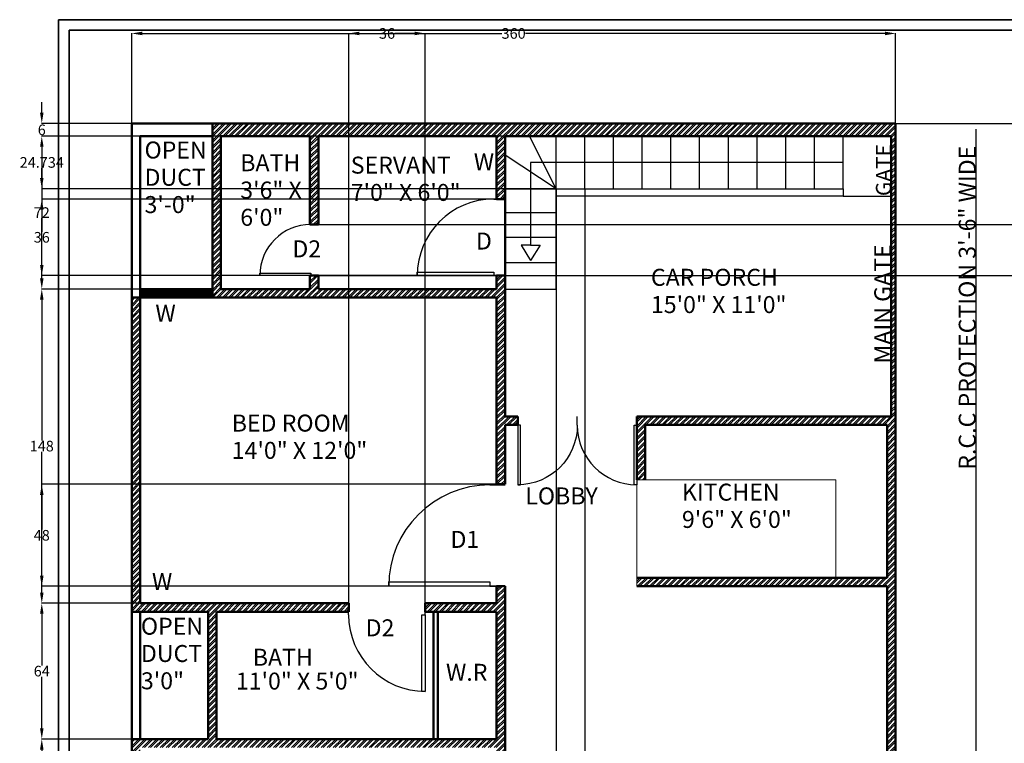
# Model space of a CAD drawing. Units: inches. Extents: x -35 to 905, y -602 to 298.
# Tile 2 of 4: x -35 to 429, y -43 to 298. Entities that reach past the tile are written whole.
import ezdxf

# ---------------------------------------------------------------- set-up
doc = ezdxf.new("R2010")
doc.units = ezdxf.units.IN
doc.header["$MEASUREMENT"] = 0
for name, color, linetype, lineweight in [('A-ANNO-DIMS', 2, 'Continuous', 18), ('A-ANNO-TEXT', 3, 'Continuous', 18), ('A-ANNO-TTLB', 7, 'Continuous', 35), ('A-AREA-IDEN', 7, 'Continuous', 18), ('A-DOOR', 4, 'Continuous', 25), ('A-FLOR-FIXT', 8, 'Continuous', 18), ('A-FLOR-STRS', 3, 'Continuous', 25), ('A-WALL', 7, 'Continuous', 50), ('A-WALL-PATT', 8, 'Continuous', 13), ('C-PROP', 1, 'Continuous', 25)]:
    doc.layers.add(name, color=color, linetype=linetype, lineweight=lineweight)
doc.styles.get("Standard").update_dxf_attribs({"font": 'arial.ttf'})
doc.dimstyles.get("Standard").update_dxf_attribs({"dimtxt": 5, "dimasz": 5, "dimexe": 0.18, "dimexo": 0.0625, "dimgap": 0.09, "dimtad": 0, "dimtih": 1, "dimtoh": 1, "dimdec": 1, "dimzin": 0, "dimdsep": 46, "dimlunit": 4, "dimtxsty": 'Standard', "dimcen": 0.09, "dimadec": 0, "dimazin": 0, "dimtfac": 1, "dimtdec": 1, "dimtofl": 0, "dimtmove": 0, "dimatfit": 3, "dimfxl": 1, "dimtolj": 1, "dimtzin": 0, "dimarcsym": 0})

# ---------------------------------------------------------------- blocks, each defined once
blk = doc.blocks.new('*U2')
for p, q in [((0, 0), (0, -6)), ((40, 0), (40, -6))]:
    blk.add_line(p, q)
blk.add_lwpolyline([(0, 0), (0, 40), (1.75, 40), (1.75, 0)], close=True)
blk.add_arc((0, 0), 40, 0, 90)
blk = doc.blocks.new('*D3')
at = {"layer": 'A-ANNO-DIMS', "color": 0, "lineweight": -2, "ltscale": 0.3, "transparency": 16777216}
for p, q in [((17.78, 249.41), (17.78, 291.93)), ((22.78, 291.75), (192.18, 291.75)), ((372.78, 291.75), (203.39, 291.75)), ((377.78, 249.41), (377.78, 291.93))]:
    blk.add_line(p, q, dxfattribs=at)
at = {"layer": 'A-ANNO-DIMS', "color": 0, "ltscale": 0.3, "transparency": 16777216}
for points in [[(22.78, 292.58), (22.78, 290.91), (17.78, 291.75)], [(372.78, 292.58), (372.78, 290.91), (377.78, 291.75)]]:
    blk.add_solid(points, dxfattribs=at)
at = {"layer": 'Defpoints', "color": 0, "ltscale": 0.3, "transparency": 16777216}
for p in [(377.78, 291.75), (17.78, 249.35), (377.78, 249.35)]:
    blk.add_point(p, dxfattribs=at)
at = {"layer": 'A-ANNO-DIMS', "color": 0, "ltscale": 0.3, "transparency": 16777216, "insert": (197.78, 291.75), "char_height": 5, "attachment_point": 5}
blk.add_mtext('\\A1;360', dxfattribs=at)
blk = doc.blocks.new('*D4')
at = {"layer": 'A-ANNO-DIMS', "color": 0, "lineweight": -2, "ltscale": 0.3, "transparency": 16777216}
for p, q in [((-24.62, 254.35), (-24.62, 259.35)), ((17.72, 249.35), (-24.8, 249.35)), ((21.72, 243.35), (-24.8, 243.35)), ((-24.62, 238.35), (-24.62, 233.35))]:
    blk.add_line(p, q, dxfattribs=at)
at = {"layer": 'A-ANNO-DIMS', "color": 0, "ltscale": 0.3, "transparency": 16777216}
for points in [[(-25.45, 254.35), (-23.78, 254.35), (-24.62, 249.35)], [(-25.45, 238.35), (-23.78, 238.35), (-24.62, 243.35)]]:
    blk.add_solid(points, dxfattribs=at)
at = {"layer": 'Defpoints', "color": 0, "ltscale": 0.3, "transparency": 16777216}
for p in [(17.78, 249.35), (-24.62, 243.35), (21.78, 243.35)]:
    blk.add_point(p, dxfattribs=at)
at = {"layer": 'A-ANNO-DIMS', "color": 0, "ltscale": 0.3, "transparency": 16777216, "insert": (-24.62, 246.35), "char_height": 5, "attachment_point": 5}
blk.add_mtext('\\A1;6', dxfattribs=at)
blk = doc.blocks.new('*D5')
at = {"layer": 'A-ANNO-DIMS', "color": 0, "lineweight": -2, "ltscale": 0.3, "transparency": 16777216}
for p, q in [((21.72, 243.35), (-24.8, 243.35)), ((-24.62, 238.35), (-24.62, 209.95)), ((-24.62, 176.35), (-24.62, 204.75)), ((21.72, 171.35), (-24.8, 171.35))]:
    blk.add_line(p, q, dxfattribs=at)
at = {"layer": 'A-ANNO-DIMS', "color": 0, "ltscale": 0.3, "transparency": 16777216}
for points in [[(-25.45, 238.35), (-23.78, 238.35), (-24.62, 243.35)], [(-25.45, 176.35), (-23.78, 176.35), (-24.62, 171.35)]]:
    blk.add_solid(points, dxfattribs=at)
at = {"layer": 'Defpoints', "color": 0, "ltscale": 0.3, "transparency": 16777216}
for p in [(21.78, 243.35), (-24.62, 171.35), (21.78, 171.35)]:
    blk.add_point(p, dxfattribs=at)
at = {"layer": 'A-ANNO-DIMS', "color": 0, "ltscale": 0.3, "transparency": 16777216, "insert": (-24.62, 207.35), "char_height": 5, "attachment_point": 5}
blk.add_mtext('\\A1;72', dxfattribs=at)
blk = doc.blocks.new('*D6')
at = {"layer": 'A-ANNO-DIMS', "color": 0, "lineweight": -2, "ltscale": 0.3, "transparency": 16777216}
for p, q in [((21.72, 171.35), (-24.8, 171.35)), ((-24.62, 166.35), (-24.62, 99.99)), ((-24.62, 28.35), (-24.62, 94.7)), ((21.72, 23.35), (-24.8, 23.35))]:
    blk.add_line(p, q, dxfattribs=at)
at = {"layer": 'A-ANNO-DIMS', "color": 0, "ltscale": 0.3, "transparency": 16777216}
for points in [[(-25.45, 166.35), (-23.78, 166.35), (-24.62, 171.35)], [(-25.45, 28.35), (-23.78, 28.35), (-24.62, 23.35)]]:
    blk.add_solid(points, dxfattribs=at)
at = {"layer": 'Defpoints', "color": 0, "ltscale": 0.3, "transparency": 16777216}
for p in [(21.78, 171.35), (-24.62, 23.35), (21.78, 23.35)]:
    blk.add_point(p, dxfattribs=at)
at = {"layer": 'A-ANNO-DIMS', "color": 0, "ltscale": 0.3, "transparency": 16777216, "insert": (-24.62, 97.35), "char_height": 5, "attachment_point": 5}
blk.add_mtext('\\A1;148', dxfattribs=at)
blk = doc.blocks.new('*D7')
at = {"layer": 'A-ANNO-DIMS', "color": 0, "lineweight": -2, "ltscale": 0.3, "transparency": 16777216}
for p, q in [((21.72, 23.35), (-24.8, 23.35)), ((-24.62, 18.35), (-24.62, -6.01)), ((-24.62, -35.65), (-24.62, -11.3)), ((21.72, -40.65), (-24.8, -40.65))]:
    blk.add_line(p, q, dxfattribs=at)
at = {"layer": 'A-ANNO-DIMS', "color": 0, "ltscale": 0.3, "transparency": 16777216}
for points in [[(-25.45, 18.35), (-23.78, 18.35), (-24.62, 23.35)], [(-25.45, -35.65), (-23.78, -35.65), (-24.62, -40.65)]]:
    blk.add_solid(points, dxfattribs=at)
at = {"layer": 'Defpoints', "color": 0, "ltscale": 0.3, "transparency": 16777216}
for p in [(21.78, 23.35), (-24.62, -40.65), (21.78, -40.65)]:
    blk.add_point(p, dxfattribs=at)
at = {"layer": 'A-ANNO-DIMS', "color": 0, "ltscale": 0.3, "transparency": 16777216, "insert": (-24.62, -8.65), "char_height": 5, "attachment_point": 5}
blk.add_mtext('\\A1;64', dxfattribs=at)
blk = doc.blocks.new('*D8')
at = {"layer": 'A-ANNO-DIMS', "color": 0, "lineweight": -2, "ltscale": 0.3, "transparency": 16777216}
for p, q in [((21.72, -40.65), (-24.8, -40.65)), ((-24.62, -45.65), (-24.62, -112.01)), ((-24.62, -183.65), (-24.62, -117.3)), ((21.72, -188.65), (-24.8, -188.65))]:
    blk.add_line(p, q, dxfattribs=at)
at = {"layer": 'A-ANNO-DIMS', "color": 0, "ltscale": 0.3, "transparency": 16777216}
for points in [[(-25.45, -45.65), (-23.78, -45.65), (-24.62, -40.65)], [(-25.45, -183.65), (-23.78, -183.65), (-24.62, -188.65)]]:
    blk.add_solid(points, dxfattribs=at)
at = {"layer": 'Defpoints', "color": 0, "ltscale": 0.3, "transparency": 16777216}
for p in [(21.78, -40.65), (-24.62, -188.65), (21.78, -188.65)]:
    blk.add_point(p, dxfattribs=at)
at = {"layer": 'A-ANNO-DIMS', "color": 0, "ltscale": 0.3, "transparency": 16777216, "insert": (-24.62, -114.65), "char_height": 5, "attachment_point": 5}
blk.add_mtext('\\A1;148', dxfattribs=at)
blk = doc.blocks.new('*D18')
at = {"layer": 'A-ANNO-DIMS', "color": 0, "lineweight": -2, "ltscale": 0.3, "transparency": 16777216}
for p, q in [((377.85, 249.35), (468.36, 249.35)), ((468.18, 244.35), (468.18, -104.51)), ((468.18, -458.65), (468.18, -109.8)), ((377.85, -463.65), (468.36, -463.65))]:
    blk.add_line(p, q, dxfattribs=at)
at = {"layer": 'A-ANNO-DIMS', "color": 0, "ltscale": 0.3, "transparency": 16777216}
for points in [[(467.35, 244.35), (469.02, 244.35), (468.18, 249.35)], [(467.35, -458.65), (469.02, -458.65), (468.18, -463.65)]]:
    blk.add_solid(points, dxfattribs=at)
at = {"layer": 'Defpoints', "color": 0, "ltscale": 0.3, "transparency": 16777216}
for p in [(377.78, 249.35), (377.78, -463.65), (468.18, -463.65)]:
    blk.add_point(p, dxfattribs=at)
at = {"layer": 'A-ANNO-DIMS', "color": 0, "ltscale": 0.3, "transparency": 16777216, "insert": (468.18, -107.15), "char_height": 5, "attachment_point": 5}
blk.add_mtext('\\A1;713', dxfattribs=at)
blk = doc.blocks.new('*D19')
at = {"layer": 'A-ANNO-DIMS', "color": 0, "lineweight": -2, "ltscale": 0.3, "transparency": 16777216}
for p, q in [((189.72, 79.35), (-24.8, 79.35)), ((-24.62, 74.35), (-24.62, 57.99)), ((-24.62, 36.35), (-24.62, 52.7)), ((189.72, 31.35), (-24.8, 31.35))]:
    blk.add_line(p, q, dxfattribs=at)
at = {"layer": 'A-ANNO-DIMS', "color": 0, "ltscale": 0.3, "transparency": 16777216}
for points in [[(-25.45, 74.35), (-23.78, 74.35), (-24.62, 79.35)], [(-25.45, 36.35), (-23.78, 36.35), (-24.62, 31.35)]]:
    blk.add_solid(points, dxfattribs=at)
at = {"layer": 'Defpoints', "color": 0, "ltscale": 0.3, "transparency": 16777216}
for p in [(-24.62, 79.35), (189.78, 79.35), (189.78, 31.35)]:
    blk.add_point(p, dxfattribs=at)
at = {"layer": 'A-ANNO-DIMS', "color": 0, "ltscale": 0.3, "transparency": 16777216, "insert": (-24.62, 55.35), "char_height": 5, "attachment_point": 5}
blk.add_mtext('\\A1;48', dxfattribs=at)
blk = doc.blocks.new('*D20')
at = {"layer": 'A-ANNO-DIMS', "color": 0, "lineweight": -2, "ltscale": 0.3, "transparency": 16777216}
for p, q in [((120.11, 23.41), (120.11, 291.93)), ((125.11, 291.75), (134.44, 291.75)), ((151.11, 291.75), (141.77, 291.75)), ((156.11, 23.41), (156.11, 291.93))]:
    blk.add_line(p, q, dxfattribs=at)
at = {"layer": 'A-ANNO-DIMS', "color": 0, "ltscale": 0.3, "transparency": 16777216}
for points in [[(125.11, 292.58), (125.11, 290.91), (120.11, 291.75)], [(151.11, 292.58), (151.11, 290.91), (156.11, 291.75)]]:
    blk.add_solid(points, dxfattribs=at)
at = {"layer": 'Defpoints', "color": 0, "ltscale": 0.3, "transparency": 16777216}
for p in [(156.11, 291.75), (120.11, 23.35), (156.11, 23.35)]:
    blk.add_point(p, dxfattribs=at)
at = {"layer": 'A-ANNO-DIMS', "color": 0, "ltscale": 0.3, "transparency": 16777216, "insert": (138.11, 291.75), "char_height": 5, "attachment_point": 5}
blk.add_mtext('\\A1;36', dxfattribs=at)
blk = doc.blocks.new('*D22')
at = {"layer": 'A-ANNO-DIMS', "color": 0, "lineweight": -2, "ltscale": 0.3, "transparency": 16777216}
for p, q in [((189.72, 213.71), (-24.8, 213.71)), ((-24.62, 208.71), (-24.62, 198.36)), ((-24.62, 182.71), (-24.62, 193.07)), ((189.72, 177.71), (-24.8, 177.71))]:
    blk.add_line(p, q, dxfattribs=at)
at = {"layer": 'A-ANNO-DIMS', "color": 0, "ltscale": 0.3, "transparency": 16777216}
for points in [[(-25.45, 208.71), (-23.78, 208.71), (-24.62, 213.71)], [(-25.45, 182.71), (-23.78, 182.71), (-24.62, 177.71)]]:
    blk.add_solid(points, dxfattribs=at)
at = {"layer": 'Defpoints', "color": 0, "ltscale": 0.3, "transparency": 16777216}
for p in [(-24.62, 213.71), (189.78, 213.71), (189.78, 177.71)]:
    blk.add_point(p, dxfattribs=at)
at = {"layer": 'A-ANNO-DIMS', "color": 0, "ltscale": 0.3, "transparency": 16777216, "insert": (-24.62, 195.71), "char_height": 5, "attachment_point": 5}
blk.add_mtext('\\A1;36', dxfattribs=at)
blk = doc.blocks.new('*D23')
at = {"layer": 'A-ANNO-DIMS', "color": 0, "lineweight": -2, "ltscale": 0.3, "transparency": 16777216}
for p, q in [((101.85, 201.71), (468.36, 201.71)), ((468.18, 196.71), (468.18, 192.31)), ((468.18, 182.71), (468.18, 187.11)), ((101.85, 177.71), (468.36, 177.71))]:
    blk.add_line(p, q, dxfattribs=at)
at = {"layer": 'A-ANNO-DIMS', "color": 0, "ltscale": 0.3, "transparency": 16777216}
for points in [[(467.35, 196.71), (469.02, 196.71), (468.18, 201.71)], [(467.35, 182.71), (469.02, 182.71), (468.18, 177.71)]]:
    blk.add_solid(points, dxfattribs=at)
at = {"layer": 'Defpoints', "color": 0, "ltscale": 0.3, "transparency": 16777216}
for p in [(101.78, 201.71), (468.18, 201.71), (101.78, 177.71)]:
    blk.add_point(p, dxfattribs=at)
at = {"layer": 'A-ANNO-DIMS', "color": 0, "ltscale": 0.3, "transparency": 16777216, "insert": (468.18, 189.71), "char_height": 5, "attachment_point": 5}
blk.add_mtext('\\A1;24', dxfattribs=at)
blk = doc.blocks.new('*D25')
at = {"layer": 'A-ANNO-DIMS', "color": 0, "lineweight": -2, "ltscale": 0.3, "transparency": 16777216}
for p, q in [((217.78, 218.55), (217.78, -564.24)), ((231.32, 218.55), (231.32, -564.24)), ((222.78, -564.06), (226.32, -564.06)), ((231.32, -564.06), (236.32, -564.06))]:
    blk.add_line(p, q, dxfattribs=at)
at = {"layer": 'A-ANNO-DIMS', "color": 0, "ltscale": 0.3, "transparency": 16777216}
for points in [[(222.78, -563.23), (222.78, -564.9), (217.78, -564.06)], [(226.32, -563.23), (226.32, -564.9), (231.32, -564.06)]]:
    blk.add_solid(points, dxfattribs=at)
at = {"layer": 'Defpoints', "color": 0, "ltscale": 0.3, "transparency": 16777216}
for p in [(217.78, 218.61), (231.32, 218.61), (231.32, -564.06)]:
    blk.add_point(p, dxfattribs=at)
at = {"layer": 'A-ANNO-DIMS', "color": 0, "ltscale": 0.3, "transparency": 16777216, "insert": (246.52, -564.06), "char_height": 5, "attachment_point": 5}
blk.add_mtext('\\A1;13.532', dxfattribs=at)
blk = doc.blocks.new('*D26')
at = {"layer": 'A-ANNO-DIMS', "color": 0, "lineweight": -2, "ltscale": 0.3, "transparency": 16777216}
for p, q in [((217.72, 243.35), (-24.8, 243.35)), ((-24.62, 238.35), (-24.62, 233.62)), ((-24.62, 223.61), (-24.62, 228.34)), ((217.72, 218.61), (-24.8, 218.61))]:
    blk.add_line(p, q, dxfattribs=at)
at = {"layer": 'A-ANNO-DIMS', "color": 0, "ltscale": 0.3, "transparency": 16777216}
for points in [[(-25.45, 238.35), (-23.78, 238.35), (-24.62, 243.35)], [(-25.45, 223.61), (-23.78, 223.61), (-24.62, 218.61)]]:
    blk.add_solid(points, dxfattribs=at)
at = {"layer": 'Defpoints', "color": 0, "ltscale": 0.3, "transparency": 16777216}
for p in [(217.78, 243.35), (-24.62, 218.61), (217.78, 218.61)]:
    blk.add_point(p, dxfattribs=at)
at = {"layer": 'A-ANNO-DIMS', "color": 0, "ltscale": 0.3, "transparency": 16777216, "insert": (-24.62, 230.98), "char_height": 5, "attachment_point": 5}
blk.add_mtext('\\A1;24.734', dxfattribs=at)

msp = doc.modelspace()

# ---------------------------------------------------------------- hatches: boundary and pattern name
at = {"layer": 'A-WALL-PATT', "ltscale": 0.3}
h = msp.add_hatch(dxfattribs=at)
h.set_pattern_fill('ANSI32', color=256, scale=5.3)
h.paths.add_polyline_path([(103.5369, -188.6534), (57.7847, -188.6534), (57.7847, -315.6534), (103.5369, -315.6534), (103.5369, -311.6534), (61.7847, -311.6534), (61.7847, -254.1534), (142.7847, -254.1534), (142.7847, -311.6534), (139.5369, -311.6534), (139.5369, -315.6534), (146.7847, -315.6534), (146.7847, -250.1534), (146.7847, -188.6534), (139.5369, -188.6534), (139.5369, -192.6534), (142.7847, -192.6534), (142.7847, -250.1534), (61.7847, -250.1534), (61.7847, -192.6534), (103.5369, -192.6534)], flags=17)
h.paths.add_polyline_path([(251.7847, -164.6534), (377.7847, -164.6534), (377.7847, 107.3466), (377.7847, 249.3466), (55.7847, 249.3466), (55.7847, 167.3466), (189.7847, 167.3466), (189.7847, 79.3466), (193.7847, 79.3466), (193.7847, 107.3466), (199.7871, 107.3466), (199.7871, 111.3466), (193.7847, 111.3466), (193.7847, 177.7106), (189.7847, 177.7106), (189.7847, 171.3466), (105.7847, 171.3466), (105.7847, 177.7106), (101.7847, 177.7106), (101.7847, 171.3466), (59.7847, 171.3466), (59.7847, 243.3466), (101.7847, 243.3466), (101.7847, 201.7106), (105.7847, 201.7106), (105.7847, 243.3466), (189.7847, 243.3466), (189.7847, 213.7106), (193.7847, 213.7106), (193.7847, 243.3466), (375.7847, 243.3466), (375.7847, 111.3466), (255.7847, 111.3466), (255.7847, 81.4115), (259.7847, 81.4115), (259.7847, 107.3466), (373.7847, 107.3466), (373.7847, 35.3466), (255.7847, 35.3466), (255.7847, 31.3466), (373.7847, 31.3466), (373.7847, -160.6534), (247.7847, -160.6534), (247.7847, -164.6534), (247.7847, -212.6534), (251.7847, -212.6534)])
h.paths.add_polyline_path([(193.7847, -311.6534), (198.4452, -307.597), (195.8191, -304.5798), (189.7847, -309.832), (185.845, -309.832), (185.845, -313.832), (189.7847, -313.832), (189.7847, -463.6534), (193.7847, -463.6534), (193.7847, -457.6052)])
h.paths.add_polyline_path([(377.7847, -260.6534), (246.2878, -260.6534), (238.9641, -267.0277), (241.5902, -270.0449), (247.7847, -264.6534), (373.7847, -264.6534), (373.7847, -463.6534), (377.7847, -463.6534)])
h.paths.add_polyline_path([(189.7847, -459.6534), (154.7661, -459.6534), (154.7661, -463.6534), (189.7847, -463.6534)])
h.paths.add_polyline_path([(65.9248, -459.6534), (21.7847, -459.6534), (21.7847, -463.6534), (65.9248, -463.6534)])
h.paths.add_polyline_path([(21.7847, -459.6534), (17.7847, -459.6534), (17.7847, -463.6534), (21.7847, -463.6534)])
h = msp.add_hatch(dxfattribs=at)
h.set_pattern_fill('ANSI32', color=256, scale=5.3)
h.paths.add_polyline_path([(193.7847, 31.3466), (189.7847, 31.3466), (189.7847, 23.3466), (156.106, 23.3466), (156.106, 19.3466), (189.7847, 19.3466), (189.7847, -40.6534), (57.7847, -40.6534), (57.7847, 19.3466), (120.106, 19.3466), (120.106, 23.3466), (21.7847, 23.3466), (21.7847, 167.3466), (17.7847, 167.3466), (17.7847, 19.3466), (53.7847, 19.3466), (53.7847, -40.6534), (17.7847, -40.6534), (17.7847, -459.6534), (21.7847, -459.6534), (21.7847, -315.6534), (21.7847, -192.6534), (21.7847, -44.6534), (189.7847, -44.6534), (189.7847, -188.6534), (189.7847, -192.6534), (193.7847, -192.6534)])

# ---------------------------------------------------------------- linework, layer by layer
at = {"layer": 'A-ANNO-TTLB', "ltscale": 0.3}
for points in [[(-16.7606, 298.2205), (890.3824, 298.2205), (890.3824, -602.0527), (-16.7606, -602.0527)], [(-11.7606, 293.2205), (885.3824, 293.2205), (885.3824, -599.6301), (-11.7606, -599.6301)]]:
    msp.add_lwpolyline(points, close=True, dxfattribs=at)
at = {"layer": 'A-FLOR-FIXT'}
for p, q in [((255.7847, 81.4115), (259.7847, 81.4115)), ((259.7847, 81.4115), (349.707, 81.4115)), ((349.707, 81.4115), (349.707, 35.3466)), ((255.7847, 35.3466), (255.7847, 31.3466))]:
    msp.add_line(p, q, dxfattribs=at)
at = {"layer": 'A-FLOR-FIXT', "ltscale": 0.3}
msp.add_line((255.7847, 81.4115), (255.7847, 35.3466), dxfattribs=at)
at = {"layer": 'A-FLOR-STRS', "ltscale": 0.3}
for p, q in [((217.7847, 218.6126), (205.3341, 243.3466)), ((217.7847, 171.3466), (217.7847, 243.3466)), ((217.7847, 218.6126), (217.7847, 243.3466)), ((231.3167, 218.6126), (231.3167, 243.3466)), ((244.8487, 218.6126), (244.8487, 243.3466)), ((258.3808, 218.6126), (258.3808, 243.3466)), ((271.9128, 218.6126), (271.9128, 243.3466)), ((285.4448, 218.6126), (285.4448, 243.3466)), ((298.9768, 218.6126), (298.9768, 243.3466)), ((312.5088, 218.6126), (312.5088, 243.3466)), ((326.0408, 218.6126), (326.0408, 243.3466)), ((339.5729, 218.6126), (339.5729, 243.3466)), ((353.1049, 218.6126), (353.1049, 243.3466)), ((217.7847, 218.6126), (193.7847, 234.4412)), ((217.7847, 230.9796), (205.7847, 230.9796)), ((205.7847, 230.9796), (205.7847, 191.9452)), ((353.1049, 230.9796), (217.7847, 230.9796)), ((193.7847, 218.6126), (217.7847, 218.6126)), ((217.7847, 218.6126), (353.1049, 218.6126)), ((353.1049, 218.6126), (353.1049, 215.1321)), ((353.1049, 215.1321), (217.7847, 215.1321)), ((353.1049, 215.1321), (375.7847, 215.1321)), ((193.7847, 207.3836), (217.7847, 207.3466)), ((193.7847, 195.7106), (217.7847, 195.7106)), ((205.7847, 191.9452), (201.3288, 191.9452)), ((201.3288, 191.9452), (205.7847, 184.8342)), ((205.7847, 191.9452), (210.2406, 191.9452)), ((210.2406, 191.9452), (205.7847, 184.8342)), ((193.7847, 183.7722), (217.7847, 183.7722)), ((193.7847, 171.3466), (217.7847, 171.3466))]:
    msp.add_line(p, q, dxfattribs=at)
at = {"layer": 'A-WALL'}
for p, q in [((17.7847, 249.3466), (17.7847, -463.6534)), ((17.7847, 249.3466), (377.7847, 249.3466)), ((55.7847, 249.3466), (55.7847, 167.3466)), ((377.7847, 249.3466), (377.7847, 107.3466)), ((21.7847, 243.3466), (55.7847, 243.3466)), ((21.7847, 243.3466), (21.7847, 171.3466)), ((59.7847, 243.3466), (59.7847, 171.3466)), ((59.7847, 243.3466), (101.7847, 243.3466)), ((101.7847, 243.3466), (101.7847, 201.7106)), ((105.7847, 243.3466), (105.7847, 201.7106)), ((105.7847, 243.3466), (189.7847, 243.3466)), ((189.7847, 243.3466), (189.7847, 213.7106)), ((193.7847, 243.3466), (193.7847, 213.7106)), ((193.7847, 243.3466), (375.7847, 243.3466)), ((375.7847, 243.3466), (375.7847, 111.3466)), ((193.7847, 213.7106), (189.7847, 213.7106)), ((101.7847, 201.7106), (105.7847, 201.7106)), ((105.7847, 177.7106), (101.7847, 177.7106)), ((101.7847, 177.7106), (101.7847, 171.3466)), ((105.7847, 177.7106), (105.7847, 171.3466)), ((189.7847, 177.7106), (193.7847, 177.7106)), ((189.7847, 177.7106), (189.7847, 171.3466)), ((193.7847, 177.7106), (193.7847, 111.3466)), ((17.7847, 167.3466), (189.7847, 167.3466)), ((21.7847, 171.3466), (55.7847, 171.3466)), ((21.7847, 167.3466), (21.7847, 23.3466)), ((59.7847, 171.3466), (101.7847, 171.3466)), ((105.7847, 171.3466), (189.7847, 171.3466)), ((189.7847, 167.3466), (189.7847, 79.3466)), ((193.7847, 111.3466), (199.7871, 111.3466)), ((193.7847, 107.3466), (199.7871, 107.3466)), ((193.7847, 107.3466), (193.7847, 79.3466)), ((199.7871, 111.3466), (199.7871, 107.3466)), ((255.7847, 111.3466), (255.7847, 81.4115)), ((255.7847, 111.3466), (375.7847, 111.3466)), ((259.7847, 107.3466), (259.7847, 81.4115)), ((259.7847, 107.3466), (373.7847, 107.3466)), ((373.7847, 107.3466), (373.7847, 35.3466)), ((377.7847, 107.3466), (377.7847, -164.6534)), ((189.7847, 79.3466), (193.7847, 79.3466)), ((255.7847, 35.3466), (373.7847, 35.3466)), ((193.7847, 31.3466), (189.7847, 31.3466)), ((189.7847, 31.3466), (189.7847, 23.3466)), ((193.7847, 31.3466), (193.7847, -192.6534)), ((255.7847, 31.3466), (373.7847, 31.3466)), ((373.7847, 31.3466), (373.7847, -160.6534)), ((21.7847, 23.3466), (120.106, 23.3466)), ((156.106, 23.3466), (189.7847, 23.3466)), ((17.7847, 19.3466), (53.7847, 19.3466)), ((21.7847, 19.3466), (21.7847, -40.6534)), ((53.7847, 19.3466), (53.7847, -40.6534)), ((57.7847, 19.3466), (57.7847, -40.6534)), ((57.7847, 19.3466), (120.106, 19.3466)), ((156.106, 19.3466), (189.7847, 19.3466)), ((160.0008, 19.3466), (160.0008, -40.6534)), ((161.9907, 19.3466), (161.9907, -40.6534)), ((189.7847, 19.3466), (189.7847, -40.6534)), ((17.7847, -40.6534), (53.7847, -40.6534)), ((57.7847, -40.6534), (189.7847, -40.6534))]:
    msp.add_line(p, q, dxfattribs=at)
at = {"layer": 'A-WALL', "ltscale": 0.3}
for p, q in [((193.7847, 213.7106), (193.7847, 177.7106)), ((21.7847, 167.3466), (21.7847, 171.3466)), ((21.7847, 170.228), (55.7847, 170.228)), ((21.7847, 169.3466), (55.7847, 169.3466)), ((21.7847, 168.3246), (55.7847, 168.3246)), ((120.106, 19.3466), (120.106, 23.3466)), ((156.106, 23.3466), (156.106, 19.3466))]:
    msp.add_line(p, q, dxfattribs=at)
at = {"layer": 'C-PROP', "ltscale": 0.3}
msp.add_line((415.5757, 246.7147), (415.5757, -498.921), dxfattribs=at)

# ---------------------------------------------------------------- block references
at = {"layer": 'A-DOOR'}
for p, xscale, yscale, zscale, rotation in [((188.3819, 177.7106), 0.9004759647644354, 0.9004759647644354, 0.9004759647644354, 90), ((102.1779, 177.7106), 0.6011270170069589, 0.6011270170069589, 0.6011270170069589, 90), ((199.7871, 107.1453), -0.700211784135817, 0.700211784135817, 0.700211784135817, 180), ((255.804, 107.1453), 0.700211784135817, 0.700211784135817, 0.700211784135817, 180), ((186.6251, 31.3466), 1.193272600612834, 1.193272600612834, 1.193272600612834, 90), ((156.106, 17.9293), 0.9028739102900063, 0.9028739102900063, 0.9028739102900063, 180)]:
    msp.add_blockref('*U2', p, dxfattribs=dict(at, xscale=xscale, yscale=yscale, zscale=zscale, rotation=rotation))

# ---------------------------------------------------------------- texts
at = {"layer": 'A-ANNO-TEXT', "ltscale": 0.3}
for s, height, p in [('GATE', 7.22209, (375.7847, 215.1321)), ('R.C.C PROTECTION 3\'-6" WIDE', 8, (415.5757, 86.2018)), ('MAIN GATE', 8, (375.7847, 136.2515))]:
    msp.add_text(s, height=height, rotation=90, dxfattribs=at).set_placement(p)
for s, p in [('W', (179.0031, 227.3078)), ('D', (180.0196, 189.9476)), ('D2', (93.492, 186.2679)), ('W', (28.9332, 155.9236)), ('D1', (168.0221, 49.3952)), ('W', (27.3046, 29.547)), ('D2', (128.0199, 7.738))]:
    msp.add_text(s, height=8, dxfattribs=at).set_placement(p)
at = {"layer": 'A-AREA-IDEN', "ltscale": 0.3}
for s, p in [('OPEN', (23.8094, 232.8327)), ('BATH', (68.9246, 226.824)), ('SERVANT', (121.0022, 225.7107)), ('DUCT', (23.8094, 219.9814)), ('3\'6" X', (68.9246, 213.9727)), ('7\'0" X 6\'0"', (121.0022, 212.8594)), ('3\'-0"', (23.8094, 207.1301)), ('6\'0"', (68.9246, 201.1214)), ('CAR PORCH', (262.4935, 172.8667)), ('15\'0" X 11\'0"', (262.4935, 160.0154)), ('BED ROOM', (64.9152, 104.1842)), ('14\'0" X 12\'0"', (64.9152, 91.3329)), ('KITCHEN', (277.1056, 71.6631)), ('LOBBY', (203.2831, 69.8811)), ('9\'6" X 6\'0"', (277.1056, 58.8118)), ('OPEN', (22.1087, 8.4961)), ('DUCT', (22.1087, -4.3552)), ('BATH', (74.8492, -6.1065)), ('3\'0"', (22.1087, -17.2065)), ('11\'0" X 5\'0"', (66.8544, -17.3421)), ('W.R', (165.9011, -13.2153))]:
    msp.add_text(s, height=8, dxfattribs=at).set_placement(p)

# ---------------------------------------------------------------- dimensions: what is measured, and where the dimension line sits
at = {"layer": 'A-ANNO-DIMS', "ltscale": 0.3}
for base, p1, p2, override, picture, middle in [((377.7847, 291.7466), (17.7847, 249.3466), (377.7847, 249.3466), {"dimdec": 0, "dimlfac": 1, "dimrnd": 0, "dimzin": 0, "dimdsep": 46, "dimlunit": 2}, '*D3', (197.7847, 291.7466)), ((156.106, 291.7466), (120.106, 23.3466), (156.106, 23.3466), {"dimdec": 0, "dimlfac": 1, "dimrnd": 0, "dimzin": 0, "dimdsep": 46, "dimlunit": 2}, '*D20', (138.106, 291.7466)), ((231.3167, -564.0622), (217.7847, 218.6126), (231.3167, 218.6126), {"dimdec": 3, "dimlfac": 1, "dimrnd": 0, "dimzin": 0, "dimdsep": 46, "dimlunit": 2}, '*D25', (246.5244, -564.0622))]:
    dim = msp.add_linear_dim(base=base, p1=p1, p2=p2, dimstyle='Standard', override=override, dxfattribs=at)
    dim.commit()
    dim.dimension.update_dxf_attribs({"geometry": picture, "text_midpoint": middle})
for base, p1, p2, override, picture, middle in [((-24.6153, 243.3466), (17.7847, 249.3466), (21.7847, 243.3466), {"dimdec": 0, "dimlfac": 1, "dimrnd": 0, "dimzin": 0, "dimdsep": 46, "dimlunit": 2}, '*D4', (-24.6153, 246.3466)), ((468.1847, -463.6534), (377.7847, 249.3466), (377.7847, -463.6534), {"dimdec": 0, "dimlfac": 1, "dimrnd": 0, "dimzin": 0, "dimdsep": 46, "dimlunit": 2}, '*D18', (468.1847, -107.1534)), ((-24.6153, 218.6126), (217.7847, 243.3466), (217.7847, 218.6126), {"dimdec": 3, "dimlfac": 1, "dimrnd": 0, "dimzin": 0, "dimdsep": 46, "dimlunit": 2}, '*D26', (-24.6153, 230.9796)), ((-24.6153, 171.3466), (21.7847, 243.3466), (21.7847, 171.3466), {"dimdec": 0, "dimlfac": 1, "dimrnd": 0, "dimzin": 0, "dimdsep": 46, "dimlunit": 2}, '*D5', (-24.6153, 207.3466)), ((-24.6153, 213.7106), (189.7847, 177.7106), (189.7847, 213.7106), {"dimdec": 0, "dimlfac": 1, "dimrnd": 0, "dimzin": 0, "dimdsep": 46, "dimlunit": 2}, '*D22', (-24.6153, 195.7106)), ((468.1847, 201.7106), (101.7847, 177.7106), (101.7847, 201.7106), {"dimdec": 0, "dimlfac": 1, "dimrnd": 0, "dimzin": 0, "dimdsep": 46, "dimlunit": 2}, '*D23', (468.1847, 189.7106)), ((-24.6153, 23.3466), (21.7847, 171.3466), (21.7847, 23.3466), {"dimdec": 0, "dimlfac": 1, "dimrnd": 0, "dimzin": 0, "dimdsep": 46, "dimlunit": 2}, '*D6', (-24.6153, 97.3466)), ((-24.6153, 79.3466), (189.7847, 31.3466), (189.7847, 79.3466), {"dimdec": 0, "dimlfac": 1, "dimrnd": 0, "dimzin": 0, "dimdsep": 46, "dimlunit": 2}, '*D19', (-24.6153, 55.3466)), ((-24.6153, -40.6534), (21.7847, 23.3466), (21.7847, -40.6534), {"dimdec": 0, "dimlfac": 1, "dimrnd": 0, "dimzin": 0, "dimdsep": 46, "dimlunit": 2}, '*D7', (-24.6153, -8.6534)), ((-24.6153, -188.6534), (21.7847, -40.6534), (21.7847, -188.6534), {"dimdec": 0, "dimlfac": 1, "dimrnd": 0, "dimzin": 0, "dimdsep": 46, "dimlunit": 2}, '*D8', (-24.6153, -114.6534))]:
    dim = msp.add_linear_dim(base=base, p1=p1, p2=p2, angle=90, dimstyle='Standard', override=override, dxfattribs=at)
    dim.commit()
    dim.dimension.update_dxf_attribs({"geometry": picture, "text_midpoint": middle})

doc.saveas('drawing.dxf')
